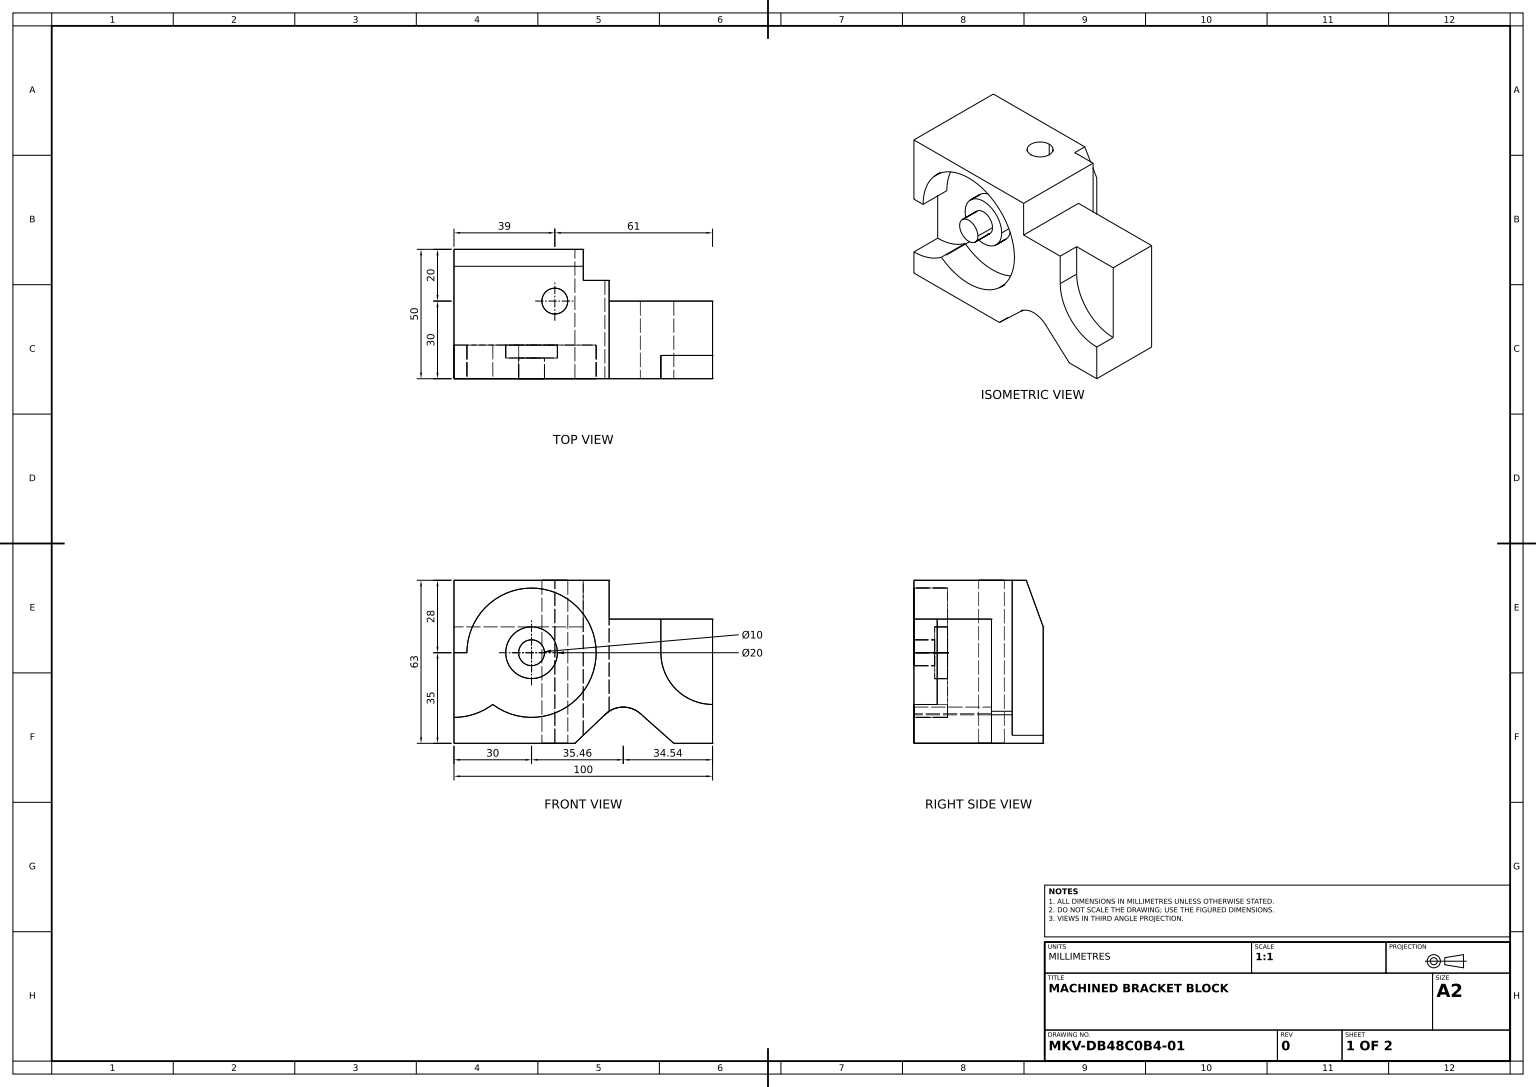
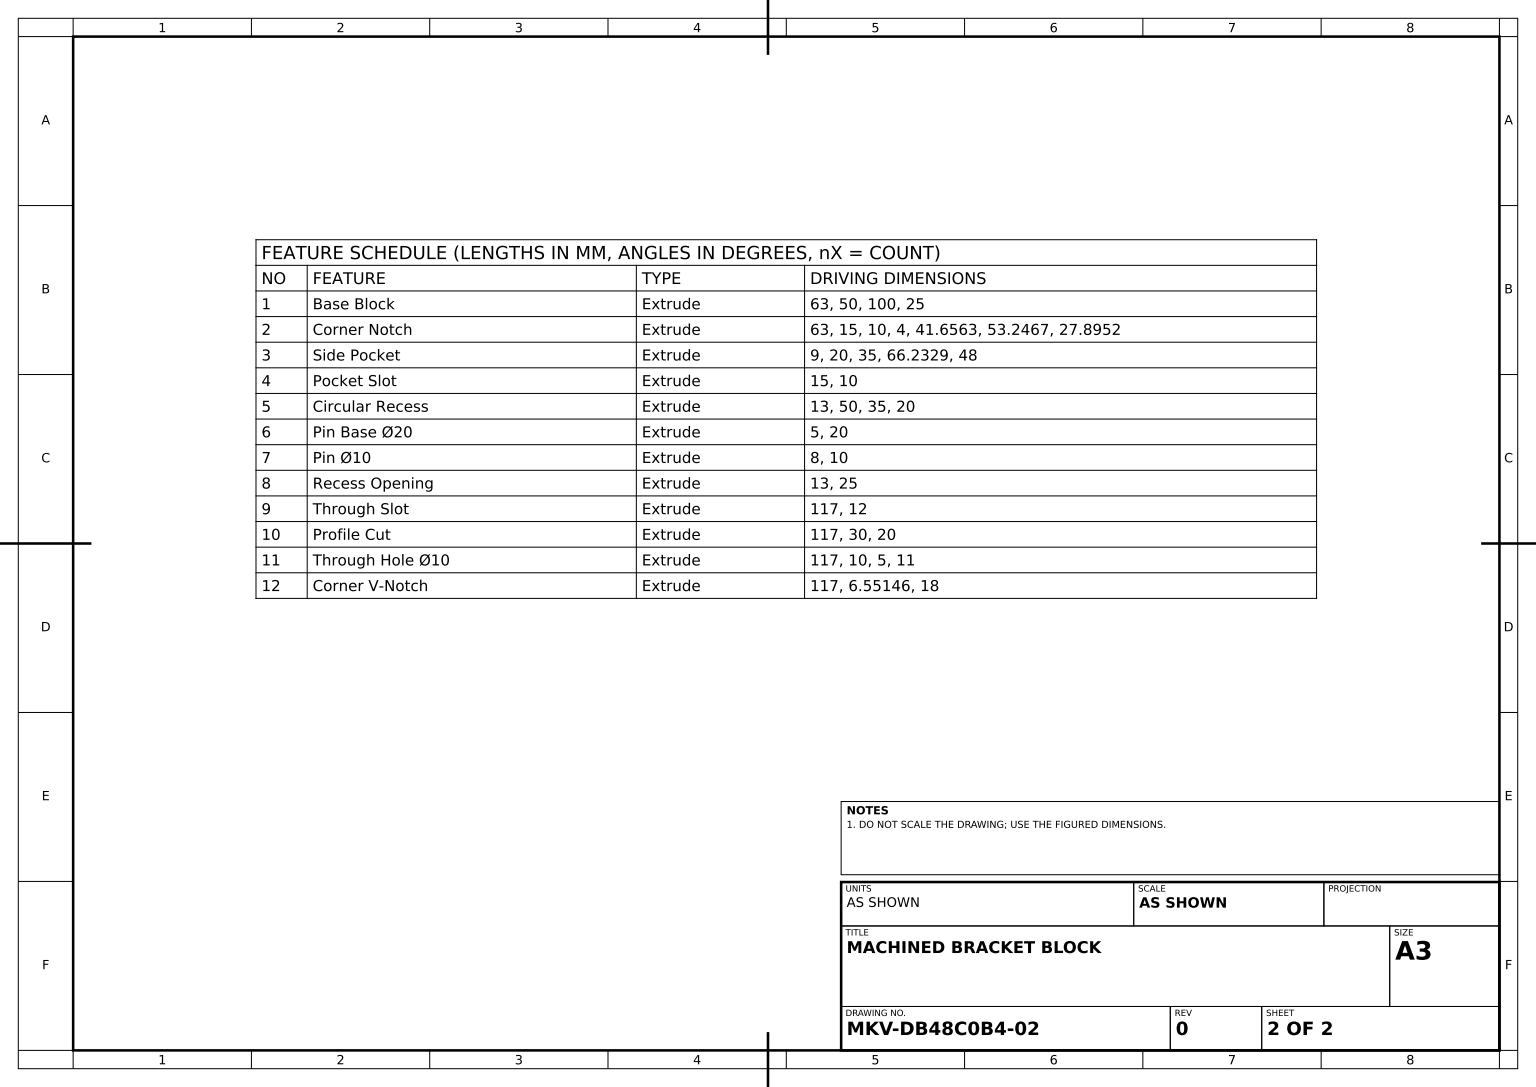
SolidWorks part; units mm, degrees
material "Plain Carbon Steel"
ref_plane "Front Plane" through (0, 0, 0) normal (0, 0, 1) x (1, 0, 0)
ref_plane "Top Plane" through (0, 0, 0) normal (0, 1, 0) x (1, 0, 0)
ref_plane "Right Plane" through (0, 0, 0) normal (1, 0, 0) x (0, 0, -1)
sketch "Base Block Sketch" plane through (0, 0, 0) normal (0, 1, 0) x (1, 0, 0)
  line L1 (50, 0) -> (50, 25)
  line L2 (50, 25) -> (-50, 25)
  line L3 (-50, 25) -> (-50, -25)
  line L4 (-50, -25) -> (50, -25)
  line L5 (50, -25) -> (50, 0)
  dimension "D1" = 50
  dimension "D2" = 100
  dimension "D3" = 25
  dimension "D4" = 50
extrude "Base Block" add sketch "Base Block Sketch" along normal blind 63
sketch "Corner Notch Sketch" plane through (0, 0, 25) normal (0, 0, 1) x (1, 0, 0)
  line L0 (50, 0) -> (35, 0)
  line L1 (-50, 0) -> (50, 0) construction
  line L2 (50, 63) -> (50, 0) construction
  line L4 (22.1048, 11.4715) -> (35, 0)
  line L5 (35, 0) -> (-3.2467, 0)
  line L6 (-3.2467, 0) -> (8.3437, 11.0273)
  arc A0 (22.1048, 11.4715) -> (8.3437, 11.0273) centre (15.4582, 4) ccw
  line M4 (-50, 0) -> (50, 0)
  dimension "D2" = 10
  dimension "D1" = 15
  dimension "D3" = 4
  dimension "D4" = 27.8952
  dimension "D6" = 41.6563
  dimension "D7" = 53.2467
extrude "Corner Notch" cut sketch "Corner Notch Sketch" against normal blind 63 contours L4 A0 L6 M4
sketch "Side Pocket Sketch" plane through (0, 0, 25) normal (0, 0, 1) x (1, 0, 0)
  line L0 (50, 0) -> (50, 35)
  line L1 (50, 63) -> (50, 0) construction
  line L2 (30, 35) -> (30, 48)
  line L3 (30, 48) -> (30, 66.2329)
  line L4 (30, 66.2329) -> (50, 66.2329)
  line L5 (50, 66.2329) -> (50, 35)
  arc A0 (30, 35) -> (50, 15) centre (50, 35) ccw
  line M5 (50, 0) -> (50, 63)
  line M6 (50, 63) -> (-50, 63)
  dimension "D1" = 20
  dimension "D2" = 35
  dimension "D3" = 66.2329
  dimension "D4" = 48
extrude "Side Pocket" cut sketch "Side Pocket Sketch" against normal blind 9 contours L2 A0 L0 L3 M5 M6 | L5 L4 L3 M6
sketch "Pocket Slot Sketch" plane through (0, 63, 0) normal (0, 1, 0) x (1, 0, 0)
  line L0 (50, -25) -> (10, -25)
  line L1 (-50, -25) -> (30, -25) construction
  line L2 (10, -25) -> (10, 25)
  line L3 (50, 25) -> (-50, 25) construction
  line L4 (10, 25) -> (50, 25)
  line L5 (50, 25) -> (50, -25)
  dimension "D1" = 10
extrude "Pocket Slot" cut sketch "Pocket Slot Sketch" against normal blind 15
sketch "Circular Recess Sketch" plane through (0, 0, 25) normal (0, 0, 1) x (1, 0, 0)
  circle A0 centre (-20, 35) radius 25
  dimension "D1" = 50
  dimension "D2" = 35
  dimension "D3" = 20
extrude "Circular Recess" cut sketch "Circular Recess Sketch" against normal blind 13
sketch "Pin Base Ø20 Sketch" plane through (0, 0, 12) normal (0, 0, 1) x (1, 0, 0)
  circle A0 centre (-20, 35) radius 10
  dimension "D1" = 20
extrude "Pin Base Ø20" add sketch "Pin Base Ø20 Sketch" along normal blind 5
sketch "Pin Ø10 Sketch" plane through (0, 0, 17) normal (0, 0, 1) x (1, 0, 0)
  circle A0 centre (-20, 35) radius 5
  dimension "D1" = 10
extrude "Pin Ø10" add sketch "Pin Ø10 Sketch" along normal blind 8
sketch "Recess Opening Sketch" plane through (0, 0, 25) normal (0, 0, 1) x (1, 0, 0)
  line L0 (-50, 35) -> (-45, 35)
  line L1 (-50, 63) -> (-50, 0) construction
  line L2 (-50, 35) -> (-50, 10)
  arc A3 (-45, 35) -> (-35, 15) centre (-20, 35) ccw
  arc A4 (-50, 10) -> (-35, 15) centre (-50, 35) ccw
  arc A5 (-45, 35) -> (-35, 15) centre (-20, 35) ccw
  circle M1 centre (-20, 35) radius 25
  line M5 (-50, 63) -> (-50, 0)
  dimension "D1" = 25
extrude "Recess Opening" cut sketch "Recess Opening Sketch" against normal blind 13 contours A4 L0 M5 M1
sketch "Through Slot Sketch" plane through (0, 63, 0) normal (0, 1, 0) x (1, 0, 0)
  line L0 (10, 25) -> (10, 13)
  line L1 (10, 25) -> (10, -25) construction
  line L2 (10, 13) -> (0, 13)
  line L3 (0, 13) -> (0, 25)
  line L4 (10, 25) -> (-50, 25) construction
  line L5 (0, 25) -> (10, 25)
  dimension "D1" = 12
extrude "Through Slot" cut sketch "Through Slot Sketch" against normal blind 117
sketch "Profile Cut Sketch" plane through (0, 48, 0) normal (0, 1, 0) x (1, 0, 0)
  line L0 (50, 25) -> (10, 25) construction
  line L2 (20, 5) -> (50, 5)
  line L3 (50, -16) -> (50, 25) construction
  line L4 (50, 5) -> (50, 25)
  line L5 (50, 25) -> (10, 25)
  line L6 (10, 25) -> (10, 5)
  line L7 (10, 13) -> (10, -25) construction
  line L8 (10, 5) -> (20, 5)
  dimension "D1" = 30
  dimension "D2" = 20
extrude "Profile Cut" cut sketch "Profile Cut Sketch" against normal blind 117
sketch "Through Hole Ø10 Sketch" plane through (0, 63, 0) normal (0, 1, 0) x (1, 0, 0)
  circle A0 centre (-11, 5) radius 5
  dimension "D1" = 10
  dimension "D2" = 5
  dimension "D3" = 11
extrude "Through Hole Ø10" cut sketch "Through Hole Ø10 Sketch" against normal blind 117
sketch "Corner V-Notch Sketch" plane through (-50, 0, 0) normal (-1, 0, 0) x (0, 0, 1)
  line L0 (-25, 63) -> (-25, 45)
  line L1 (-25, 63) -> (-25, 0) construction
  line L2 (-25, 45) -> (-18.4485, 63)
  line L3 (-25, 63) -> (-18.4485, 63)
  line L4 (-25, 63) -> (25, 63) construction
  dimension "D1" = 6.5515
  dimension "D2" = 18
extrude "Corner V-Notch" cut sketch "Corner V-Notch Sketch" against normal blind 117
